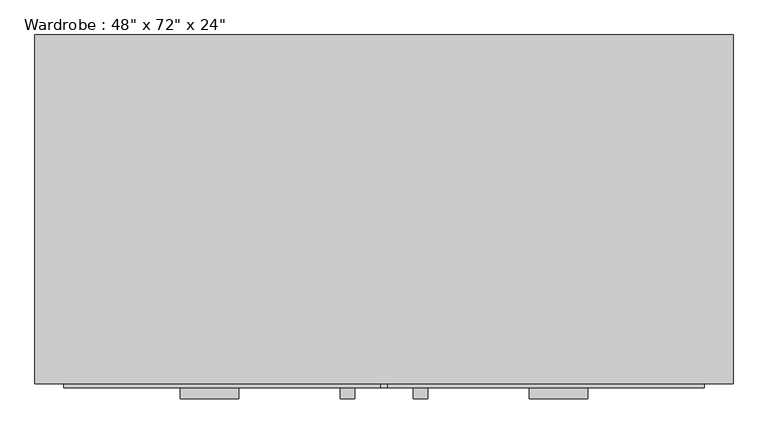
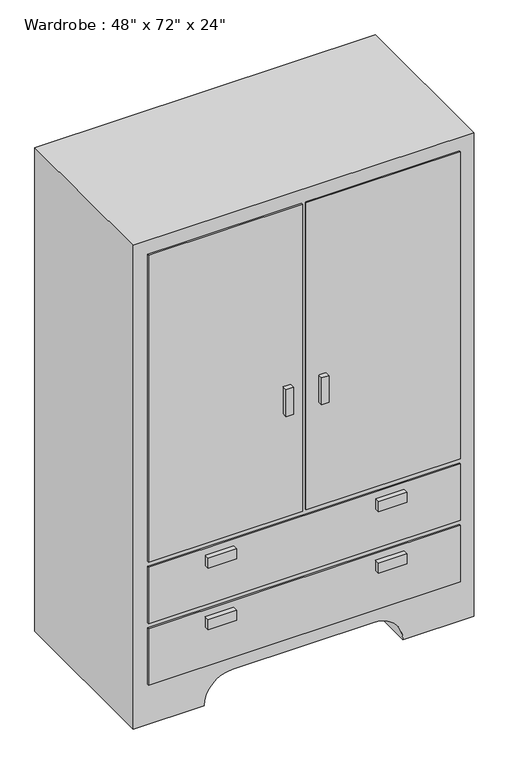
"""IFC4 building model written with IfcOpenShell, lengths in millimetres: furniture geometry."""

from ifc_helpers import new_model, si_unit, point, frame, frame_2d, origin, place, context, project, spatial, polyline, circle_curve, trimmed, segment, composite_curve, outline, extrude, source, transform, mapped, element, save


def furniture_82e269c4(model_context):
    return source(origin(), model_context, "Body", "SweptSolid", [
        extrude(outline(composite_curve([segment(polyline([(0.0, 340.4067402), (1828.8, 340.4067402), (1828.8, -878.7932598), (0.0, -878.7932598), (0.0, -624.7932598)]), True, "CONTINUOUS"), segment(trimmed(circle_curve(frame_2d((0.0, -523.1932598)), 101.6), [point((0.0, -624.7932598))], [point((101.6, -523.1932598))], True, "CARTESIAN"), True, "CONTINUOUS"), segment(polyline([(101.6, -523.1932598), (101.6, -15.1932598)]), True, "CONTINUOUS"), segment(trimmed(circle_curve(frame_2d((0.0, -15.1932598)), 101.6), [point((101.6, -15.1932598))], [point((0.0, 86.4067402))], True, "CARTESIAN"), True, "CONTINUOUS"), segment(polyline([(0.0, 86.4067402), (0.0, 340.4067402)]), True, "CONTINUOUS")], self_intersect=False)), frame((0.0, -888.5388096, 0.0), z_axis=(0.0, 1.0, 0.0), x_axis=(0.0, 0.0, 1.0)), (0.0, 0.0, 1.0), 609.6),
        extrude(outline(polyline([(289.6067402, -894.8888096), (-827.9932598, -894.8888096), (-827.9932598, -888.5388096), (289.6067402, -888.5388096), (289.6067402, -894.8888096)])), frame((0.0, 0.0, 384.6285714), z_axis=(0.0, 0.0, 1.0), x_axis=(1.0, 0.0, 0.0)), (0.0, 0.0, 1.0), 213.1785714),
        extrude(outline(polyline([(289.6067402, -894.8888096), (-827.9932598, -894.8888096), (-827.9932598, -888.5388096), (289.6067402, -888.5388096), (289.6067402, -894.8888096)])), frame((0.0, 0.0, 152.4), z_axis=(0.0, 0.0, 1.0), x_axis=(1.0, 0.0, 0.0)), (0.0, 0.0, 1.0), 213.1785714),
        extrude(outline(polyline([(-275.5432598, -894.8888096), (-827.9932598, -894.8888096), (-827.9932598, -888.5388096), (-275.5432598, -888.5388096), (-275.5432598, -894.8888096)])), frame((0.0, 0.0, 616.8571429), z_axis=(0.0, 0.0, 1.0), x_axis=(1.0, 0.0, 0.0)), (0.0, 0.0, 1.0), 1161.1428571),
        extrude(outline(polyline([(289.6067402, -894.8888096), (-262.8432598, -894.8888096), (-262.8432598, -888.5388096), (289.6067402, -888.5388096), (289.6067402, -894.8888096)])), frame((0.0, 0.0, 616.8571429), z_axis=(0.0, 0.0, 1.0), x_axis=(1.0, 0.0, 0.0)), (0.0, 0.0, 1.0), 1161.1428571),
        extrude(outline(polyline([(-319.9932598, -913.9388096), (-345.3932598, -913.9388096), (-345.3932598, -894.8888096), (-319.9932598, -894.8888096), (-319.9932598, -913.9388096)])), frame((0.0, 0.0, 1010.5571429), z_axis=(0.0, 0.0, 1.0), x_axis=(1.0, 0.0, 0.0)), (0.0, 0.0, 1.0), 101.6),
        extrude(outline(polyline([(-192.9932598, -913.9388096), (-218.3932598, -913.9388096), (-218.3932598, -894.8888096), (-192.9932598, -894.8888096), (-192.9932598, -913.9388096)])), frame((0.0, 0.0, 1010.5571429), z_axis=(0.0, 0.0, 1.0), x_axis=(1.0, 0.0, 0.0)), (0.0, 0.0, 1.0), 101.6),
        extrude(outline(polyline([(-523.1932598, -913.9388096), (-624.7932598, -913.9388096), (-624.7932598, -894.8888096), (-523.1932598, -894.8888096), (-523.1932598, -913.9388096)])), frame((0.0, 0.0, 534.3071429), z_axis=(0.0, 0.0, 1.0), x_axis=(1.0, 0.0, 0.0)), (0.0, 0.0, 1.0), 38.1),
        extrude(outline(polyline([(86.4067402, -913.9388096), (-15.1932598, -913.9388096), (-15.1932598, -894.8888096), (86.4067402, -894.8888096), (86.4067402, -913.9388096)])), frame((0.0, 0.0, 534.3071429), z_axis=(0.0, 0.0, 1.0), x_axis=(1.0, 0.0, 0.0)), (0.0, 0.0, 1.0), 38.1),
        extrude(outline(polyline([(86.4067402, -913.9388096), (-15.1932598, -913.9388096), (-15.1932598, -894.8888096), (86.4067402, -894.8888096), (86.4067402, -913.9388096)])), frame((0.0, 0.0, 302.0785714), z_axis=(0.0, 0.0, 1.0), x_axis=(1.0, 0.0, 0.0)), (0.0, 0.0, 1.0), 38.1),
        extrude(outline(polyline([(-523.1932598, -913.9388096), (-624.7932598, -913.9388096), (-624.7932598, -894.8888096), (-523.1932598, -894.8888096), (-523.1932598, -913.9388096)])), frame((0.0, 0.0, 302.0785714), z_axis=(0.0, 0.0, 1.0), x_axis=(1.0, 0.0, 0.0)), (0.0, 0.0, 1.0), 38.1),
    ])


if __name__ == "__main__":
    model = new_model("IFC4")
    model_context = context("Model", 3, world=origin())
    ifc_project = project(units=[si_unit("LENGTHUNIT", "METRE", prefix="MILLI")], contexts=[model_context])
    site = spatial("IfcSite", under=ifc_project)
    building = spatial("IfcBuilding", under=site)
    placement = place(None, origin())
    furniture_shape = furniture_82e269c4(model_context)
    element("IfcFurniture", 1, ObjectType="Wardrobe : 48\" x 72\" x 24\"", at=placement, inside=building, context=model_context, shape_type="MappedRepresentation", body=[
        mapped(furniture_shape, transform((0.0, 0.0, 0.0), x_axis=(1.0, 0.0, 0.0), y_axis=(0.0, 1.0, 0.0), z_axis=(0.0, 0.0, 1.0))),
    ])
    save(model, "model.ifc")

# Revit data of these elements
# Type "Wardrobe : 48\" x 72\" x 24\""
#   Assembly Code = "E2020200"
#   Depth = 2' - 0"
#   Height = 6' - 0"
#   Width = 4' - 0"
#   Material = Wood - Mahogany
#   Default Elevation = 0
# Element 1 (IfcFurniture, "Wardrobe : 48\" x 72\" x 24\"")
#   Materials on its faces: "Wood - Mahogany"
# Materials
#   "Wood - Mahogany": colour RGB 138 86 45, transparency 0
